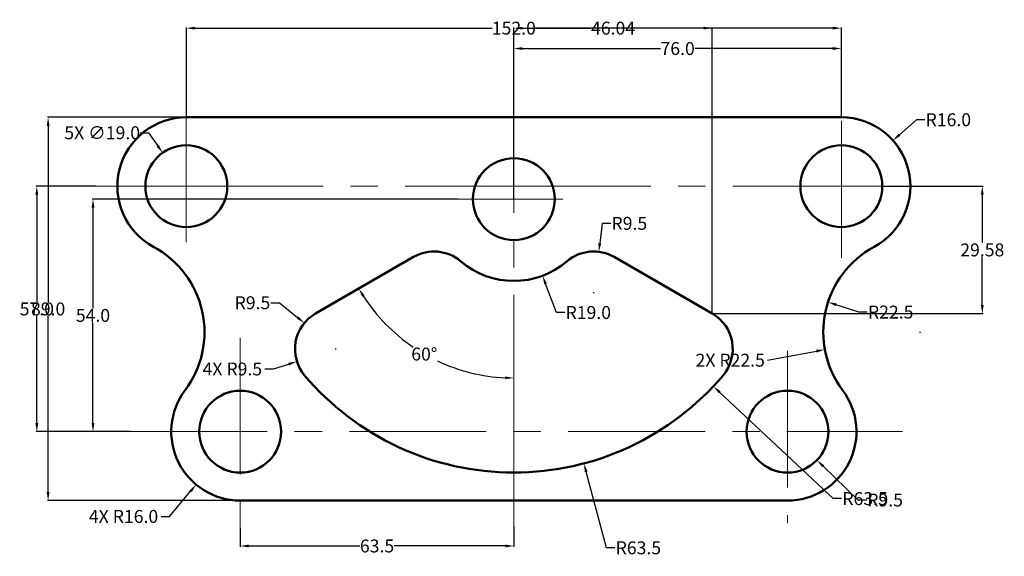
# Model space of a CAD drawing. Units: inches. Extents: x 175 to 404, y 108 to 233.
import ezdxf

# ---------------------------------------------------------------- set-up
doc = ezdxf.new("R2010")
doc.units = ezdxf.units.IN
doc.header["$MEASUREMENT"] = 0
doc.linetypes.add('CENTER', pattern=[50.8, 31.75, -6.35, 6.35, -6.35])
for name, color, linetype, lineweight in [('M-CNTR', 4, 'CENTER', 18), ('M-DIMS', 2, 'Continuous', 25), ('M-OUTL', 7, 'Continuous', 50)]:
    doc.layers.add(name, color=color, linetype=linetype, lineweight=lineweight)
doc.styles.get("Standard").update_dxf_attribs({"font": 'arial.ttf'})
doc.dimstyles.get("Standard").update_dxf_attribs({"dimtxt": 3, "dimasz": 2, "dimexe": 0.18, "dimexo": 0.0625, "dimgap": 0.09, "dimtad": 0, "dimtih": 1, "dimtoh": 1, "dimdec": 1, "dimzin": 0, "dimdsep": 46, "dimtxsty": 'Standard', "dimcen": 0.09, "dimclrd": 1, "dimclre": 1, "dimadec": 0, "dimazin": 0, "dimtfac": 1, "dimtdec": 1, "dimtofl": 0, "dimtmove": 0, "dimatfit": 3, "dimfxl": 1, "dimtolj": 1, "dimtzin": 0, "dimarcsym": 0})

# ---------------------------------------------------------------- blocks, each defined once
blk = doc.blocks.new('*D1')
at = {"layer": 'Defpoints', "color": 0, "transparency": 16777216}
for p in [(365.73, 226.37), (365.73, 220), (289.73, 218.02)]:
    blk.add_point(p, dxfattribs=at)
at = {"layer": 'M-DIMS', "color": 0, "lineweight": -2, "transparency": 16777216}
for p, q in [((289.73, 218.08), (289.73, 226.55)), ((291.73, 226.37), (323.76, 226.37)), ((363.73, 226.37), (331.7, 226.37)), ((365.73, 220.06), (365.73, 226.55))]:
    blk.add_line(p, q, dxfattribs=at)
at = {"layer": 'M-DIMS', "color": 0, "transparency": 16777216}
for points in [[(291.73, 226.7), (291.73, 226.04), (289.73, 226.37)], [(363.73, 226.7), (363.73, 226.04), (365.73, 226.37)]]:
    blk.add_solid(points, dxfattribs=at)
at = {"layer": 'M-DIMS', "color": 0, "transparency": 16777216, "insert": (327.73, 226.37), "char_height": 3, "attachment_point": 5}
blk.add_mtext('\\A1;76.0', dxfattribs=at)
blk = doc.blocks.new('*D2')
at = {"layer": 'Defpoints', "color": 0, "transparency": 16777216}
for p in [(362.62, 167.49), (384.01, 160.52)]:
    blk.add_point(p, dxfattribs=at)
at = {"layer": 'M-DIMS', "color": 0, "lineweight": -2, "transparency": 16777216}
for p, q in [((369.74, 165.17), (364.52, 166.87)), ((371.74, 165.17), (369.74, 165.17))]:
    blk.add_line(p, q, dxfattribs=at)
at = {"layer": 'M-DIMS', "color": 0, "transparency": 16777216}
blk.add_solid([(364.62, 167.19), (364.42, 166.55), (362.62, 167.49)], dxfattribs=at)
at = {"layer": 'M-DIMS', "color": 0, "transparency": 16777216, "insert": (377.17, 165.17), "char_height": 3, "attachment_point": 5}
blk.add_mtext('\\A1;R22.5', dxfattribs=at)
blk = doc.blocks.new('*D3')
at = {"layer": 'Defpoints', "color": 0, "transparency": 16777216}
for p in [(353.23, 137.4), (360.05, 130.79)]:
    blk.add_point(p, dxfattribs=at)
at = {"layer": 'M-DIMS', "color": 0, "lineweight": -2, "transparency": 16777216}
for p, q in [((353.14, 137.4), (353.32, 137.4)), ((353.23, 137.31), (353.23, 137.49)), ((369.6, 121.53), (361.48, 129.4)), ((371.6, 121.53), (369.6, 121.53))]:
    blk.add_line(p, q, dxfattribs=at)
at = {"layer": 'M-DIMS', "color": 0, "transparency": 16777216}
blk.add_solid([(361.72, 129.64), (361.25, 129.16), (360.05, 130.79)], dxfattribs=at)
at = {"layer": 'M-DIMS', "color": 0, "transparency": 16777216, "insert": (375.87, 121.53), "char_height": 3, "attachment_point": 5}
blk.add_mtext('\\A1;R9.5', dxfattribs=at)
blk = doc.blocks.new('*D4')
at = {"layer": 'Defpoints', "color": 0, "transparency": 16777216}
for p in [(289.73, 191.4), (306, 130.02)]:
    blk.add_point(p, dxfattribs=at)
at = {"layer": 'M-DIMS', "color": 0, "lineweight": -2, "transparency": 16777216}
for p, q in [((289.64, 191.4), (289.82, 191.4)), ((289.73, 191.31), (289.73, 191.49)), ((311.19, 110.42), (306.51, 128.09)), ((313.19, 110.42), (311.19, 110.42))]:
    blk.add_line(p, q, dxfattribs=at)
at = {"layer": 'M-DIMS', "color": 0, "transparency": 16777216}
blk.add_solid([(306.83, 128.17), (306.19, 128), (306, 130.02)], dxfattribs=at)
at = {"layer": 'M-DIMS', "color": 0, "transparency": 16777216, "insert": (318.62, 110.42), "char_height": 3, "attachment_point": 5}
blk.add_mtext('\\A1;R63.5', dxfattribs=at)
blk = doc.blocks.new('*D5')
at = {"layer": 'Defpoints', "color": 0, "transparency": 16777216}
for p in [(226.23, 115.08), (289.73, 115.47), (226.23, 110.86)]:
    blk.add_point(p, dxfattribs=at)
at = {"layer": 'M-DIMS', "color": 0, "lineweight": -2, "transparency": 16777216}
for p, q in [((226.23, 115.02), (226.23, 110.68)), ((289.73, 115.4), (289.73, 110.68)), ((228.23, 110.86), (253.97, 110.86)), ((287.73, 110.86), (261.98, 110.86))]:
    blk.add_line(p, q, dxfattribs=at)
at = {"layer": 'M-DIMS', "color": 0, "transparency": 16777216}
for points in [[(228.23, 111.19), (228.23, 110.52), (226.23, 110.86)], [(287.73, 111.19), (287.73, 110.52), (289.73, 110.86)]]:
    blk.add_solid(points, dxfattribs=at)
at = {"layer": 'M-DIMS', "color": 0, "transparency": 16777216, "insert": (257.98, 110.86), "char_height": 3, "attachment_point": 5}
blk.add_mtext('\\A1;63.5', dxfattribs=at)
blk = doc.blocks.new('*D6')
at = {"layer": 'Defpoints', "color": 0, "transparency": 16777216}
for p in [(289.73, 191.4), (266.46, 177.97), (243.69, 164.82), (263.02, 159.58), (289.73, 137.4)]:
    blk.add_point(p, dxfattribs=at)
at = {"layer": 'M-DIMS', "color": 0, "lineweight": -2, "transparency": 16777216}
for start, end in [(212.7585, 235.7908), (244.735, 267.2415)]:
    blk.add_arc((289.73, 191.4), 41.55, start, end, dxfattribs=at)
at = {"layer": 'M-DIMS', "color": 0, "transparency": 16777216}
for points in [[(254.5, 168.75), (255.07, 169.1), (253.75, 170.63)], [(287.74, 150.24), (287.72, 149.57), (289.73, 149.86)]]:
    blk.add_solid(points, dxfattribs=at)
at = {"layer": 'M-DIMS', "color": 0, "transparency": 16777216, "insert": (268.95, 155.42), "char_height": 3, "attachment_point": 5}
blk.add_mtext('\\A1;60°', dxfattribs=at)
blk = doc.blocks.new('*D7')
at = {"layer": 'Defpoints', "color": 0, "transparency": 16777216}
for p in [(289.73, 191.4), (296.39, 173.61)]:
    blk.add_point(p, dxfattribs=at)
at = {"layer": 'M-DIMS', "color": 0, "lineweight": -2, "transparency": 16777216}
for p, q in [((289.64, 191.4), (289.82, 191.4)), ((289.73, 191.31), (289.73, 191.49)), ((299.59, 165.07), (297.09, 171.74)), ((301.59, 165.07), (299.59, 165.07))]:
    blk.add_line(p, q, dxfattribs=at)
at = {"layer": 'M-DIMS', "color": 0, "transparency": 16777216}
blk.add_solid([(297.4, 171.85), (296.78, 171.62), (296.39, 173.61)], dxfattribs=at)
at = {"layer": 'M-DIMS', "color": 0, "transparency": 16777216, "insert": (307, 165.07), "char_height": 3, "attachment_point": 5}
blk.add_mtext('\\A1;R19.0', dxfattribs=at)
blk = doc.blocks.new('*D8')
at = {"layer": 'Defpoints', "color": 0, "transparency": 16777216}
for p in [(309.43, 179.17), (308.25, 169.74)]:
    blk.add_point(p, dxfattribs=at)
at = {"layer": 'M-DIMS', "color": 0, "lineweight": -2, "transparency": 16777216}
for p, q in [((310.25, 185.77), (309.67, 181.15)), ((312.25, 185.77), (310.25, 185.77)), ((308.16, 169.74), (308.34, 169.74)), ((308.25, 169.65), (308.25, 169.83))]:
    blk.add_line(p, q, dxfattribs=at)
at = {"layer": 'M-DIMS', "color": 0, "transparency": 16777216}
blk.add_solid([(309.34, 181.19), (310, 181.11), (309.43, 179.17)], dxfattribs=at)
at = {"layer": 'M-DIMS', "color": 0, "transparency": 16777216, "insert": (316.52, 185.77), "char_height": 3, "attachment_point": 5}
blk.add_mtext('\\A1;R9.5', dxfattribs=at)
blk = doc.blocks.new('*D9')
at = {"layer": 'Defpoints', "color": 0, "transparency": 16777216}
for p in [(377.7, 205.02), (365.73, 194.4)]:
    blk.add_point(p, dxfattribs=at)
at = {"layer": 'M-DIMS', "color": 0, "lineweight": -2, "transparency": 16777216}
for p, q in [((383.12, 209.83), (379.2, 206.34)), ((385.12, 209.83), (383.12, 209.83)), ((365.64, 194.4), (365.82, 194.4)), ((365.73, 194.31), (365.73, 194.49))]:
    blk.add_line(p, q, dxfattribs=at)
at = {"layer": 'M-DIMS', "color": 0, "transparency": 16777216}
blk.add_solid([(378.98, 206.59), (379.42, 206.09), (377.7, 205.02)], dxfattribs=at)
at = {"layer": 'M-DIMS', "color": 0, "transparency": 16777216, "insert": (390.54, 209.83), "char_height": 3, "attachment_point": 5}
blk.add_mtext('\\A1;R16.0', dxfattribs=at)
blk = doc.blocks.new('*D10')
at = {"layer": 'Defpoints', "color": 0, "transparency": 16777216}
for p in [(241.1, 162.62), (248.44, 156.6)]:
    blk.add_point(p, dxfattribs=at)
at = {"layer": 'M-DIMS', "color": 0, "lineweight": -2, "transparency": 16777216}
for p, q in [((233.34, 167.34), (235.34, 167.34)), ((235.34, 167.34), (239.55, 163.89)), ((248.35, 156.6), (248.53, 156.6)), ((248.44, 156.51), (248.44, 156.69))]:
    blk.add_line(p, q, dxfattribs=at)
at = {"layer": 'M-DIMS', "color": 0, "transparency": 16777216}
blk.add_solid([(239.76, 164.15), (239.34, 163.63), (241.1, 162.62)], dxfattribs=at)
at = {"layer": 'M-DIMS', "color": 0, "transparency": 16777216, "insert": (229.07, 167.34), "char_height": 3, "attachment_point": 5}
blk.add_mtext('\\A1;R9.5', dxfattribs=at)
blk = doc.blocks.new('*D11')
at = {"layer": 'Defpoints', "color": 0, "transparency": 16777216}
for p in [(192.76, 194.4), (179.04, 137.4), (200.77, 137.4)]:
    blk.add_point(p, dxfattribs=at)
at = {"layer": 'M-DIMS', "color": 0, "lineweight": -2, "transparency": 16777216}
for p, q in [((192.7, 194.4), (178.86, 194.4)), ((179.04, 192.4), (179.04, 167.52)), ((179.04, 139.4), (179.04, 164.28)), ((200.7, 137.4), (178.86, 137.4))]:
    blk.add_line(p, q, dxfattribs=at)
at = {"layer": 'M-DIMS', "color": 0, "transparency": 16777216}
for points in [[(178.7, 192.4), (179.37, 192.4), (179.04, 194.4)], [(178.7, 139.4), (179.37, 139.4), (179.04, 137.4)]]:
    blk.add_solid(points, dxfattribs=at)
at = {"layer": 'M-DIMS', "color": 0, "transparency": 16777216, "insert": (179.04, 165.9), "char_height": 3, "attachment_point": 5}
blk.add_mtext('\\A1;57.0', dxfattribs=at)
blk = doc.blocks.new('*D12')
at = {"layer": 'Defpoints', "color": 0, "transparency": 16777216}
for p in [(276.88, 191.4), (192.07, 137.4), (200.77, 137.4)]:
    blk.add_point(p, dxfattribs=at)
at = {"layer": 'M-DIMS', "color": 0, "lineweight": -2, "transparency": 16777216}
for p, q in [((276.81, 191.4), (191.89, 191.4)), ((192.07, 189.4), (192.07, 166.02)), ((192.07, 139.4), (192.07, 162.78)), ((200.7, 137.4), (191.89, 137.4))]:
    blk.add_line(p, q, dxfattribs=at)
at = {"layer": 'M-DIMS', "color": 0, "transparency": 16777216}
for points in [[(191.74, 189.4), (192.41, 189.4), (192.07, 191.4)], [(191.74, 139.4), (192.41, 139.4), (192.07, 137.4)]]:
    blk.add_solid(points, dxfattribs=at)
at = {"layer": 'M-DIMS', "color": 0, "transparency": 16777216, "insert": (192.07, 164.4), "char_height": 3, "attachment_point": 5}
blk.add_mtext('\\A1;54.0', dxfattribs=at)
blk = doc.blocks.new('HOLE-D19')
blk.add_circle((9.5, 9.5), 9.5)
blk = doc.blocks.new('*D14')
at = {"layer": 'Defpoints', "color": 0, "transparency": 16777216}
for p in [(181.66, 210.4), (213.73, 210.4), (226.23, 121.4)]:
    blk.add_point(p, dxfattribs=at)
at = {"layer": 'M-DIMS', "color": 1, "lineweight": -2, "transparency": 16777216}
for p, q in [((213.66, 210.4), (181.48, 210.4)), ((181.66, 208.4), (181.66, 167.52)), ((181.66, 123.4), (181.66, 164.28)), ((226.16, 121.4), (181.48, 121.4))]:
    blk.add_line(p, q, dxfattribs=at)
at = {"layer": 'M-DIMS', "color": 1, "transparency": 16777216}
for points in [[(181.32, 208.4), (181.99, 208.4), (181.66, 210.4)], [(181.32, 123.4), (181.99, 123.4), (181.66, 121.4)]]:
    blk.add_solid(points, dxfattribs=at)
at = {"layer": 'M-DIMS', "color": 0, "transparency": 16777216, "insert": (181.66, 165.9), "char_height": 3, "attachment_point": 5}
blk.add_mtext('\\A1;89.0', dxfattribs=at)
blk = doc.blocks.new('*D15')
at = {"layer": 'Defpoints', "color": 0, "transparency": 16777216}
for p in [(365.73, 231.1), (213.73, 210.4), (365.73, 210.4)]:
    blk.add_point(p, dxfattribs=at)
at = {"layer": 'M-DIMS', "color": 1, "lineweight": -2, "transparency": 16777216}
for p, q in [((213.73, 210.47), (213.73, 231.28)), ((215.73, 231.1), (284.72, 231.1)), ((363.73, 231.1), (294.73, 231.1)), ((365.73, 210.47), (365.73, 231.28))]:
    blk.add_line(p, q, dxfattribs=at)
at = {"layer": 'M-DIMS', "color": 1, "transparency": 16777216}
for points in [[(215.73, 231.43), (215.73, 230.77), (213.73, 231.1)], [(363.73, 231.43), (363.73, 230.77), (365.73, 231.1)]]:
    blk.add_solid(points, dxfattribs=at)
at = {"layer": 'M-DIMS', "color": 0, "transparency": 16777216, "insert": (289.73, 231.1), "char_height": 3, "attachment_point": 5}
blk.add_mtext('\\A1;152.0', dxfattribs=at)
blk = doc.blocks.new('*D16')
at = {"layer": 'Defpoints', "color": 0, "transparency": 16777216}
for p in [(289.73, 231.1), (289.73, 191.4), (335.76, 164.82)]:
    blk.add_point(p, dxfattribs=at)
at = {"layer": 'M-DIMS', "color": 1, "lineweight": -2, "transparency": 16777216}
for p, q in [((289.73, 191.47), (289.73, 231.28)), ((291.73, 231.1), (307.54, 231.1)), ((333.76, 231.1), (317.95, 231.1)), ((335.76, 164.89), (335.76, 231.28))]:
    blk.add_line(p, q, dxfattribs=at)
at = {"layer": 'M-DIMS', "color": 1, "transparency": 16777216}
for points in [[(291.73, 231.43), (291.73, 230.77), (289.73, 231.1)], [(333.76, 231.43), (333.76, 230.77), (335.76, 231.1)]]:
    blk.add_solid(points, dxfattribs=at)
at = {"layer": 'M-DIMS', "color": 0, "transparency": 16777216, "insert": (312.75, 231.1), "char_height": 3, "attachment_point": 5}
blk.add_mtext('\\A1;46.04', dxfattribs=at)
blk = doc.blocks.new('*D17')
at = {"layer": 'Defpoints', "color": 0, "transparency": 16777216}
for p in [(375.23, 194.4), (398.42, 194.4), (335.76, 164.82)]:
    blk.add_point(p, dxfattribs=at)
at = {"layer": 'M-DIMS', "color": 1, "lineweight": -2, "transparency": 16777216}
for p, q in [((375.29, 194.4), (398.6, 194.4)), ((398.42, 192.4), (398.42, 181.24)), ((398.42, 166.82), (398.42, 177.99)), ((335.83, 164.82), (398.6, 164.82))]:
    blk.add_line(p, q, dxfattribs=at)
at = {"layer": 'M-DIMS', "color": 1, "transparency": 16777216}
for points in [[(398.08, 192.4), (398.75, 192.4), (398.42, 194.4)], [(398.08, 166.82), (398.75, 166.82), (398.42, 164.82)]]:
    blk.add_solid(points, dxfattribs=at)
at = {"layer": 'M-DIMS', "color": 0, "transparency": 16777216, "insert": (398.42, 179.61), "char_height": 3, "attachment_point": 5}
blk.add_mtext('\\A1;29.58', dxfattribs=at)
blk = doc.blocks.new('*D18')
at = {"layer": 'Defpoints', "color": 0, "transparency": 16777216}
for p in [(289.73, 191.4), (336.02, 147.93)]:
    blk.add_point(p, dxfattribs=at)
at = {"layer": 'M-DIMS', "color": 1, "lineweight": -2, "transparency": 16777216}
for p, q in [((289.64, 191.4), (289.82, 191.4)), ((289.73, 191.31), (289.73, 191.49)), ((363.79, 121.85), (337.47, 146.57)), ((365.79, 121.85), (363.79, 121.85))]:
    blk.add_line(p, q, dxfattribs=at)
at = {"layer": 'M-DIMS', "color": 1, "transparency": 16777216}
blk.add_solid([(337.7, 146.81), (337.25, 146.32), (336.02, 147.93)], dxfattribs=at)
at = {"layer": 'M-DIMS', "color": 0, "transparency": 16777216, "insert": (371.22, 121.85), "char_height": 3, "attachment_point": 5}
blk.add_mtext('\\A1;R63.5', dxfattribs=at)
blk = doc.blocks.new('*D19')
at = {"layer": 'Defpoints', "color": 0, "transparency": 16777216}
for p in [(248.44, 156.6), (239.39, 153.7)]:
    blk.add_point(p, dxfattribs=at)
at = {"layer": 'M-DIMS', "color": 1, "lineweight": -2, "transparency": 16777216}
for p, q in [((248.35, 156.6), (248.53, 156.6)), ((248.44, 156.51), (248.44, 156.69)), ((233.97, 151.96), (237.49, 153.09)), ((231.97, 151.96), (233.97, 151.96))]:
    blk.add_line(p, q, dxfattribs=at)
at = {"layer": 'M-DIMS', "color": 1, "transparency": 16777216}
blk.add_solid([(237.39, 153.41), (237.59, 152.77), (239.39, 153.7)], dxfattribs=at)
at = {"layer": 'M-DIMS', "color": 0, "transparency": 16777216, "insert": (224.41, 151.96), "char_height": 3, "attachment_point": 5}
blk.add_mtext('\\A1;4X R9.5', dxfattribs=at)
blk = doc.blocks.new('*D20')
at = {"layer": 'Defpoints', "color": 0, "transparency": 16777216}
for p in [(384.01, 160.52), (361.88, 156.45)]:
    blk.add_point(p, dxfattribs=at)
at = {"layer": 'M-DIMS', "color": 1, "lineweight": -2, "transparency": 16777216}
for p, q in [((383.92, 160.52), (384.1, 160.52)), ((384.01, 160.43), (384.01, 160.61)), ((348.61, 154), (359.92, 156.08))]:
    blk.add_line(p, q, dxfattribs=at)
at = {"layer": 'M-DIMS', "color": 1, "transparency": 16777216}
blk.add_solid([(359.86, 156.41), (359.98, 155.76), (361.88, 156.45)], dxfattribs=at)
at = {"layer": 'M-DIMS', "color": 0, "transparency": 16777216, "insert": (339.93, 154), "char_height": 3, "attachment_point": 5}
blk.add_mtext('\\A1;2X R22.5', dxfattribs=at)
blk = doc.blocks.new('*D21')
at = {"layer": 'Defpoints', "color": 0, "transparency": 16777216}
for p in [(226.23, 137.4), (216, 125.1)]:
    blk.add_point(p, dxfattribs=at)
at = {"layer": 'M-DIMS', "color": 1, "lineweight": -2, "transparency": 16777216}
for p, q in [((226.14, 137.4), (226.32, 137.4)), ((226.23, 137.31), (226.23, 137.49)), ((209.86, 117.72), (214.72, 123.56)), ((207.86, 117.72), (209.86, 117.72))]:
    blk.add_line(p, q, dxfattribs=at)
at = {"layer": 'M-DIMS', "color": 1, "transparency": 16777216}
blk.add_solid([(214.46, 123.77), (214.98, 123.35), (216, 125.1)], dxfattribs=at)
at = {"layer": 'M-DIMS', "color": 0, "transparency": 16777216, "insert": (199.16, 117.72), "char_height": 3, "attachment_point": 5}
blk.add_mtext('\\A1;4X R16.0', dxfattribs=at)
blk = doc.blocks.new('*D22')
at = {"layer": 'Defpoints', "color": 0, "transparency": 16777216}
for p in [(208.24, 202.16), (219.21, 186.65)]:
    blk.add_point(p, dxfattribs=at)
at = {"layer": 'M-DIMS', "color": 1, "lineweight": -2, "transparency": 16777216}
for p, q in [((202.95, 206.81), (204.95, 206.81)), ((204.95, 206.81), (207.09, 203.79)), ((213.64, 194.4), (213.82, 194.4)), ((213.73, 194.31), (213.73, 194.49))]:
    blk.add_line(p, q, dxfattribs=at)
at = {"layer": 'M-DIMS', "color": 1, "transparency": 16777216}
blk.add_solid([(207.36, 203.99), (206.82, 203.6), (208.24, 202.16)], dxfattribs=at)
at = {"layer": 'M-DIMS', "color": 0, "transparency": 16777216, "insert": (194.2, 206.81), "char_height": 3, "attachment_point": 5}
blk.add_mtext('\\A1;5X ∅19.0', dxfattribs=at)

msp = doc.modelspace()

# ---------------------------------------------------------------- linework, layer by layer
at = {"layer": 'M-CNTR'}
for p, q in [((213.727, 181.412), (213.727, 219.682)), ((365.727, 177.799), (365.727, 219.999)), ((301.118, 191.403), (276.876, 191.403)), ((226.227, 159.173), (226.227, 115.084)), ((353.227, 156.146), (353.227, 116.137)), ((200.766, 137.403), (379.909, 137.403))]:
    msp.add_line(p, q, dxfattribs=at)
for points in [[(192.758, 194.403), (213.727, 194.403), (289.727, 194.403), (289.727, 218.021)], [(289.727, 115.466), (289.727, 137.403), (289.727, 191.403), (289.727, 194.403), (365.727, 194.403), (387.318, 194.403)]]:
    msp.add_lwpolyline(points, dxfattribs=at)
at = {"layer": 'M-OUTL'}
for p, q in [((213.727, 210.403), (365.727, 210.403)), ((266.457, 177.968), (243.691, 164.824)), ((312.997, 177.968), (335.763, 164.824)), ((226.227, 121.403), (353.227, 121.403))]:
    msp.add_line(p, q, dxfattribs=at)
for centre, radius, start, end in [((213.727, 194.403), 16, 90, 241.64416), ((365.727, 194.403), 16, 298.35584, 90), ((195.442, 160.522), 22.5, 323.09396, 61.64416), ((271.207, 169.741), 9.5, 49.47122, 120), ((308.247, 169.741), 9.5, 60, 130.52878), ((384.013, 160.522), 22.5, 118.35584, 216.90604), ((289.727, 191.403), 19, 229.47122, 310.52878), ((248.441, 156.597), 9.5, 120, 220.13255), ((331.013, 156.597), 9.5, 319.86745, 60), ((289.727, 191.403), 63.5, 220.13255, 319.86745), ((226.227, 137.403), 16, 143.09396, 270), ((353.227, 137.403), 16, 270, 36.90604)]:
    msp.add_arc(centre, radius, start, end, dxfattribs=at)

# ---------------------------------------------------------------- block references
for p in [(204.227, 184.903), (356.227, 184.903), (280.227, 181.903), (216.727, 127.903), (343.727, 127.903)]:
    msp.add_blockref('HOLE-D19', p, dxfattribs=at)

# ---------------------------------------------------------------- dimensions: what is measured, and where the dimension line sits
at = {"layer": 'M-DIMS'}
for base, p1, p2, override, picture, middle in [((365.727, 231.099), (213.727, 210.403), (365.727, 210.403), {"dimdec": 1, "dimlfac": 1, "dimrnd": 0, "dimzin": 0, "dimdsep": 46, "dimlunit": 2}, '*D15', (289.727, 231.099)), ((289.727, 231.099), (335.763, 164.824), (289.727, 191.403), {"dimdec": 2, "dimlfac": 1, "dimrnd": 0, "dimzin": 0, "dimdsep": 46, "dimlunit": 2}, '*D16', (312.745, 231.099)), ((365.727, 226.37), (289.727, 218.021), (365.727, 219.999), {"dimclrd": 0, "dimclre": 0, "dimclrt": 0}, '*D1', (327.727, 226.37)), ((226.227, 110.856), (289.727, 115.466), (226.227, 115.084), {"dimclrd": 0, "dimclre": 0, "dimclrt": 0}, '*D5', (257.977, 110.856))]:
    dim = msp.add_linear_dim(base=base, p1=p1, p2=p2, dimstyle='Standard', override=override, dxfattribs=at)
    dim.commit()
    dim.dimension.update_dxf_attribs({"geometry": picture, "text_midpoint": middle})
for base, p1, p2, override, picture, middle in [((181.658, 210.403), (226.227, 121.403), (213.727, 210.403), {"dimdec": 1, "dimlfac": 1, "dimrnd": 0, "dimzin": 0, "dimdsep": 46, "dimlunit": 2}, '*D14', (181.658, 165.903)), ((179.038, 137.403), (192.758, 194.403), (200.766, 137.403), {"dimclrd": 0, "dimclre": 0, "dimclrt": 0}, '*D11', (179.038, 165.903)), ((398.418, 194.403), (335.763, 164.824), (375.227, 194.403), {"dimdec": 2, "dimlfac": 1, "dimrnd": 0, "dimzin": 0, "dimdsep": 46, "dimlunit": 2}, '*D17', (398.418, 179.614)), ((192.072, 137.403), (276.876, 191.403), (200.766, 137.403), {"dimclrd": 0, "dimclre": 0, "dimclrt": 0}, '*D12', (192.072, 164.403))]:
    dim = msp.add_linear_dim(base=base, p1=p1, p2=p2, angle=90, dimstyle='Standard', override=override, dxfattribs=at)
    dim.commit()
    dim.dimension.update_dxf_attribs({"geometry": picture, "text_midpoint": middle})
dim = msp.add_diameter_dim_2p(p1=(219.212, 186.646), p2=(208.243, 202.16), text='5X <>', dimstyle='Standard', override={"dimdec": 1, "dimlfac": 1, "dimrnd": 0, "dimzin": 0, "dimdsep": 46, "dimlunit": 2}, dxfattribs=at)
dim.commit()
dim.dimension.update_dxf_attribs({"geometry": '*D22', "text_midpoint": (194.196, 206.814), "dimtype": 163})
for center, mpoint, override, picture, middle in [((365.727, 194.403), (377.7, 205.017), {"dimclrd": 0, "dimclre": 0, "dimclrt": 0}, '*D9', (390.541, 209.826)), ((289.727, 191.403), (305.996, 130.022), {"dimclrd": 0, "dimclre": 0, "dimclrt": 0}, '*D4', (318.624, 110.421)), ((289.727, 191.403), (296.39, 173.61), {"dimclrd": 0, "dimclre": 0, "dimclrt": 0}, '*D7', (307.005, 165.07)), ((289.727, 191.403), (336.017, 147.934), {"dimdec": 1, "dimlfac": 1, "dimrnd": 0, "dimzin": 0, "dimdsep": 46, "dimlunit": 2}, '*D18', (371.224, 121.853)), ((308.247, 169.741), (309.426, 179.167), {"dimclrd": 0, "dimclre": 0, "dimclrt": 0}, '*D8', (316.519, 185.771)), ((248.441, 156.597), (241.096, 162.621), {"dimclrd": 0, "dimclre": 0, "dimclrt": 0}, '*D10', (229.071, 167.342)), ((384.013, 160.522), (362.619, 167.49), {"dimclrd": 0, "dimclre": 0, "dimclrt": 0}, '*D2', (377.175, 165.17)), ((353.227, 137.403), (360.048, 130.791), {"dimclrd": 0, "dimclre": 0, "dimclrt": 0}, '*D3', (375.867, 121.532))]:
    dim = msp.add_radius_dim(center=center, mpoint=mpoint, dimstyle='Standard', override=override, dxfattribs=at)
    dim.commit()
    dim.dimension.update_dxf_attribs({"geometry": picture, "text_midpoint": middle, "dimtype": 164})
dim = msp.add_angular_dim_2l(base=(263.022, 159.578), line1=((289.727, 137.403), (289.727, 191.403)), line2=((266.457, 177.968), (243.691, 164.824)), dimstyle='Standard', override={"dimclrd": 0, "dimclre": 0, "dimclrt": 0}, dxfattribs=at)
dim.commit()
dim.dimension.update_dxf_attribs({"geometry": '*D6', "text_midpoint": (268.955, 155.424)})
for center, mpoint, text, picture, middle in [((384.013, 160.522), (361.885, 156.447), '2X <>', '*D20', (348.608, 154.002)), ((248.441, 156.597), (239.394, 153.698), '4X <>', '*D19', (224.415, 151.959)), ((226.227, 137.403), (215.999, 125.099), '4X <>', '*D21', (199.162, 117.717))]:
    dim = msp.add_radius_dim(center=center, mpoint=mpoint, text=text, dimstyle='Standard', override={"dimdec": 1, "dimlfac": 1, "dimrnd": 0, "dimzin": 0, "dimdsep": 46, "dimlunit": 2}, dxfattribs=at)
    dim.commit()
    dim.dimension.update_dxf_attribs({"geometry": picture, "text_midpoint": middle, "dimtype": 164})

doc.saveas('drawing.dxf')
